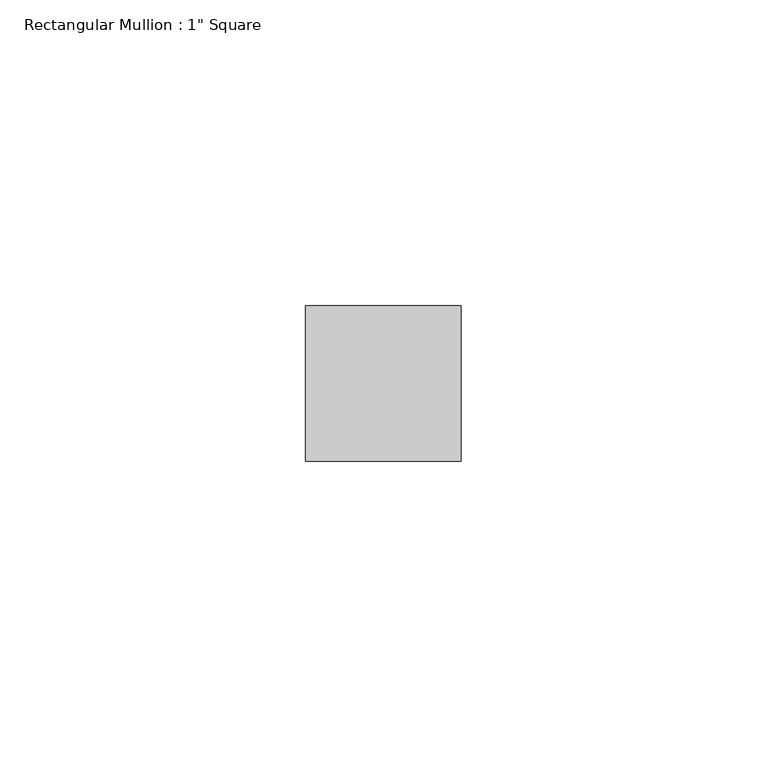
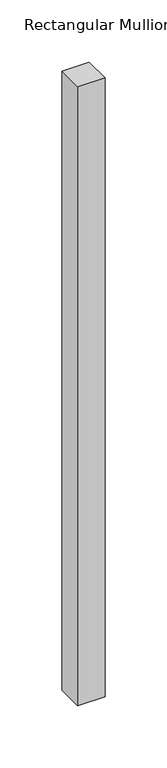
"""IFC4 building model written with IfcOpenShell, lengths in millimetres: member geometry."""

from ifc_helpers import new_model, si_unit, frame, origin, place, context, project, spatial, polyline, outline, extrude, source, transform, mapped, element, save


def member_3e1f1dd8(model_context):
    return source(origin(), model_context, "Body", "SweptSolid", [
        extrude(outline(polyline([(12.7, 12.7), (12.7, -12.7), (-12.7, -12.7), (-12.7, 12.7), (12.7, 12.7)])), frame((0.0, 0.0, -609.6), z_axis=(0.0, 0.0, 1.0), x_axis=(1.0, 0.0, 0.0)), (0.0, 0.0, 1.0), 609.6),
    ])


if __name__ == "__main__":
    model = new_model("IFC4")
    model_context = context("Model", 3, world=origin())
    ifc_project = project(units=[si_unit("LENGTHUNIT", "METRE", prefix="MILLI")], contexts=[model_context])
    site = spatial("IfcSite", under=ifc_project)
    building = spatial("IfcBuilding", under=site)
    placement = place(None, origin())
    member_shape = member_3e1f1dd8(model_context)
    element("IfcMember", 1, ObjectType="Rectangular Mullion : 1\" Square", at=placement, inside=building, context=model_context, shape_type="MappedRepresentation", body=[
        mapped(member_shape, transform((0.0, 0.0, 0.0), x_axis=(1.0, 0.0, 0.0), y_axis=(0.0, 1.0, 0.0), z_axis=(0.0, 0.0, 1.0))),
    ])
    save(model, "model.ifc")

# Revit data of these elements
# Type "Rectangular Mullion : 1\" Square"
#   built-in parameter 1007304 = 0.0833333 (stored number, unit not read)
#   built-in parameter 1007301 = 0.0416667 (stored number, unit not read)
#   built-in parameter 1007300 = 0.0416667 (stored number, unit not read)
# Element 1 (IfcMember, "Rectangular Mullion : 1\" Square")
#   Materials on its faces: "Aluminum"
# Materials
#   "Aluminum": class "Metal", colour RGB 247 247 247, transparency 0, Description = "Aluminum 6061", Cost = 0
